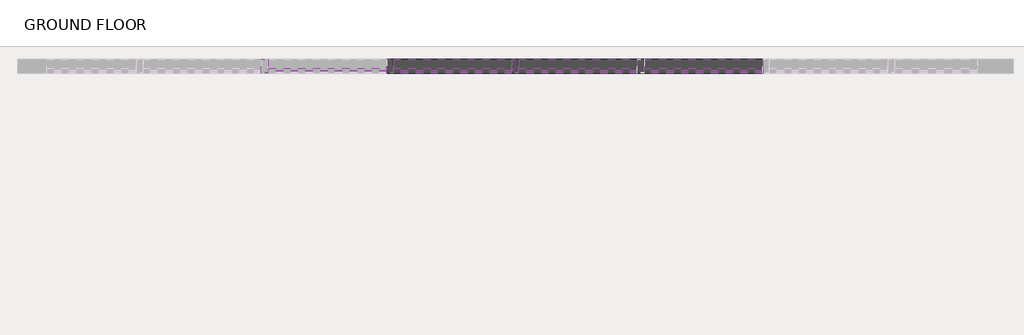
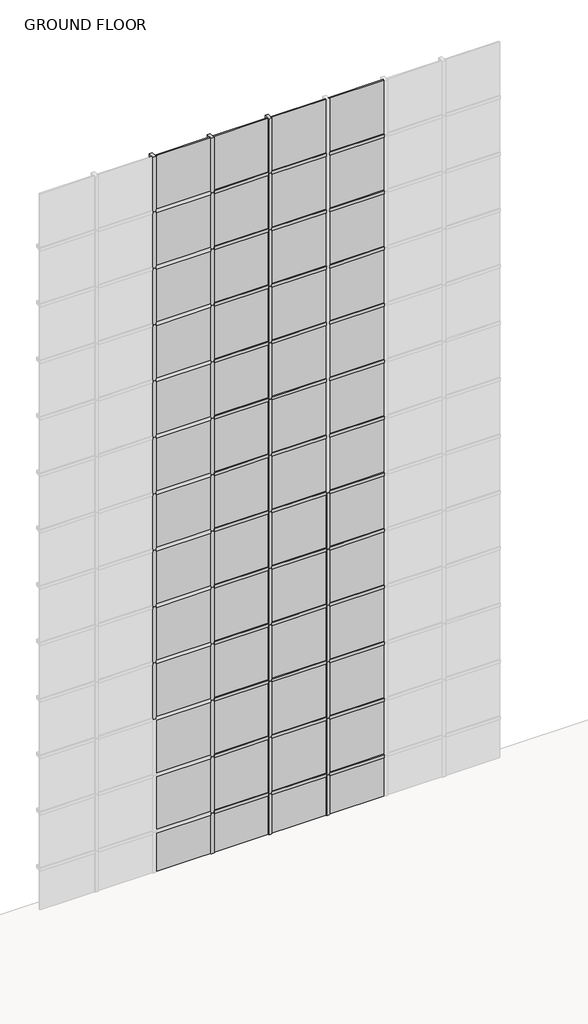
# One storey, part 10 of 16: 78 members, 52 plates.
"""IFC4 building model written with IfcOpenShell, lengths in millimetres."""

from ifc_helpers import new_model, si_unit, origin, place, context, project, spatial, transform, mapped, element, save
from components import member_d518c94e, member_b860638c, member_31fee25f, system_panel_glazed_5cba32e5

model = new_model("IFC4")

# Units and contexts
model_context = context("Model", 3, world=origin())
ifc_project = project(units=[si_unit("LENGTHUNIT", "METRE", prefix="MILLI")], contexts=[model_context])

# Site, building, storey
site = spatial("IfcSite", under=ifc_project)
building = spatial("IfcBuilding", under=site)
storey = spatial("IfcBuildingStorey", under=building, Name="GROUND FLOOR", Elevation=0.0)

# Members
placement = place(None, origin())
member_shape = member_d518c94e(model_context)
element("IfcMember", 1, ObjectType="Rectangular Mullion : 2.5\" x 5\" rectangular", at=placement, inside=storey, context=model_context, shape_type="MappedRepresentation", body=[
    mapped(member_shape, transform((-966.6171381, 6370.2261968, 1168.8884615), x_axis=(0.0, 0.0, 1.0), y_axis=(0.0, 1.0, 0.0), z_axis=(-1.0, 0.0, 0.0))),
])
element("IfcMember", 2, ObjectType="Rectangular Mullion : 2.5\" x 5\" rectangular", at=placement, inside=storey, context=model_context, shape_type="MappedRepresentation", body=[
    mapped(member_shape, transform((-2132.0863688, 6370.2261968, 1168.8884615), x_axis=(0.0, 0.0, 1.0), y_axis=(0.0, 1.0, 0.0), z_axis=(-1.0, 0.0, 0.0))),
])
element("IfcMember", 3, ObjectType="Rectangular Mullion : 2.5\" x 5\" rectangular", at=placement, inside=storey, context=model_context, shape_type="MappedRepresentation", body=[
    mapped(member_shape, transform((-3297.5555995, 6370.2261968, 1168.8884615), x_axis=(0.0, 0.0, 1.0), y_axis=(0.0, 1.0, 0.0), z_axis=(-1.0, 0.0, 0.0))),
])
element("IfcMember", 4, ObjectType="Rectangular Mullion : 2.5\" x 5\" rectangular", at=placement, inside=storey, context=model_context, shape_type="MappedRepresentation", body=[
    mapped(member_shape, transform((-966.6171381, 6370.2261968, 2369.5269231), x_axis=(0.0, 0.0, 1.0), y_axis=(0.0, 1.0, 0.0), z_axis=(-1.0, 0.0, 0.0))),
])
element("IfcMember", 5, ObjectType="Rectangular Mullion : 2.5\" x 5\" rectangular", at=placement, inside=storey, context=model_context, shape_type="MappedRepresentation", body=[
    mapped(member_shape, transform((-2132.0863688, 6370.2261968, 2369.5269231), x_axis=(0.0, 0.0, 1.0), y_axis=(0.0, 1.0, 0.0), z_axis=(-1.0, 0.0, 0.0))),
])
element("IfcMember", 6, ObjectType="Rectangular Mullion : 2.5\" x 5\" rectangular", at=placement, inside=storey, context=model_context, shape_type="MappedRepresentation", body=[
    mapped(member_shape, transform((-3297.5555995, 6370.2261968, 2369.5269231), x_axis=(0.0, 0.0, 1.0), y_axis=(0.0, 1.0, 0.0), z_axis=(-1.0, 0.0, 0.0))),
])
element("IfcMember", 7, ObjectType="Rectangular Mullion : 2.5\" x 5\" rectangular", at=placement, inside=storey, context=model_context, shape_type="MappedRepresentation", body=[
    mapped(member_shape, transform((-966.6171381, 6370.2261968, 3570.1653846), x_axis=(0.0, 0.0, 1.0), y_axis=(0.0, 1.0, 0.0), z_axis=(-1.0, 0.0, 0.0))),
])
element("IfcMember", 8, ObjectType="Rectangular Mullion : 2.5\" x 5\" rectangular", at=placement, inside=storey, context=model_context, shape_type="MappedRepresentation", body=[
    mapped(member_shape, transform((-2132.0863688, 6370.2261968, 3570.1653846), x_axis=(0.0, 0.0, 1.0), y_axis=(0.0, 1.0, 0.0), z_axis=(-1.0, 0.0, 0.0))),
])
element("IfcMember", 9, ObjectType="Rectangular Mullion : 2.5\" x 5\" rectangular", at=placement, inside=storey, context=model_context, shape_type="MappedRepresentation", body=[
    mapped(member_shape, transform((-3297.5555995, 6370.2261968, 3570.1653846), x_axis=(0.0, 0.0, 1.0), y_axis=(0.0, 1.0, 0.0), z_axis=(-1.0, 0.0, 0.0))),
])
element("IfcMember", 10, ObjectType="Rectangular Mullion : 2.5\" x 5\" rectangular", at=placement, inside=storey, context=model_context, shape_type="MappedRepresentation", body=[
    mapped(member_shape, transform((-966.6171381, 6370.2261968, 4770.8038462), x_axis=(0.0, 0.0, 1.0), y_axis=(0.0, 1.0, 0.0), z_axis=(-1.0, 0.0, 0.0))),
])
element("IfcMember", 11, ObjectType="Rectangular Mullion : 2.5\" x 5\" rectangular", at=placement, inside=storey, context=model_context, shape_type="MappedRepresentation", body=[
    mapped(member_shape, transform((-2132.0863688, 6370.2261968, 4770.8038462), x_axis=(0.0, 0.0, 1.0), y_axis=(0.0, 1.0, 0.0), z_axis=(-1.0, 0.0, 0.0))),
])
element("IfcMember", 12, ObjectType="Rectangular Mullion : 2.5\" x 5\" rectangular", at=placement, inside=storey, context=model_context, shape_type="MappedRepresentation", body=[
    mapped(member_shape, transform((-3297.5555995, 6370.2261968, 4770.8038462), x_axis=(0.0, 0.0, 1.0), y_axis=(0.0, 1.0, 0.0), z_axis=(-1.0, 0.0, 0.0))),
])
element("IfcMember", 13, ObjectType="Rectangular Mullion : 2.5\" x 5\" rectangular", at=placement, inside=storey, context=model_context, shape_type="MappedRepresentation", body=[
    mapped(member_shape, transform((-966.6171381, 6370.2261968, 5971.4423077), x_axis=(0.0, 0.0, 1.0), y_axis=(0.0, 1.0, 0.0), z_axis=(-1.0, 0.0, 0.0))),
])
element("IfcMember", 14, ObjectType="Rectangular Mullion : 2.5\" x 5\" rectangular", at=placement, inside=storey, context=model_context, shape_type="MappedRepresentation", body=[
    mapped(member_shape, transform((-2132.0863688, 6370.2261968, 5971.4423077), x_axis=(0.0, 0.0, 1.0), y_axis=(0.0, 1.0, 0.0), z_axis=(-1.0, 0.0, 0.0))),
])
element("IfcMember", 15, ObjectType="Rectangular Mullion : 2.5\" x 5\" rectangular", at=placement, inside=storey, context=model_context, shape_type="MappedRepresentation", body=[
    mapped(member_shape, transform((-3297.5555995, 6370.2261968, 5971.4423077), x_axis=(0.0, 0.0, 1.0), y_axis=(0.0, 1.0, 0.0), z_axis=(-1.0, 0.0, 0.0))),
])
element("IfcMember", 16, ObjectType="Rectangular Mullion : 2.5\" x 5\" rectangular", at=placement, inside=storey, context=model_context, shape_type="MappedRepresentation", body=[
    mapped(member_shape, transform((-966.6171381, 6370.2261968, 7172.0807692), x_axis=(0.0, 0.0, 1.0), y_axis=(0.0, 1.0, 0.0), z_axis=(-1.0, 0.0, 0.0))),
])
element("IfcMember", 17, ObjectType="Rectangular Mullion : 2.5\" x 5\" rectangular", at=placement, inside=storey, context=model_context, shape_type="MappedRepresentation", body=[
    mapped(member_shape, transform((-2132.0863688, 6370.2261968, 7172.0807692), x_axis=(0.0, 0.0, 1.0), y_axis=(0.0, 1.0, 0.0), z_axis=(-1.0, 0.0, 0.0))),
])
element("IfcMember", 18, ObjectType="Rectangular Mullion : 2.5\" x 5\" rectangular", at=placement, inside=storey, context=model_context, shape_type="MappedRepresentation", body=[
    mapped(member_shape, transform((-3297.5555995, 6370.2261968, 7172.0807692), x_axis=(0.0, 0.0, 1.0), y_axis=(0.0, 1.0, 0.0), z_axis=(-1.0, 0.0, 0.0))),
])
element("IfcMember", 19, ObjectType="Rectangular Mullion : 2.5\" x 5\" rectangular", at=placement, inside=storey, context=model_context, shape_type="MappedRepresentation", body=[
    mapped(member_shape, transform((-966.6171381, 6370.2261968, 8372.7192308), x_axis=(0.0, 0.0, 1.0), y_axis=(0.0, 1.0, 0.0), z_axis=(-1.0, 0.0, 0.0))),
])
element("IfcMember", 20, ObjectType="Rectangular Mullion : 2.5\" x 5\" rectangular", at=placement, inside=storey, context=model_context, shape_type="MappedRepresentation", body=[
    mapped(member_shape, transform((-2132.0863688, 6370.2261968, 8372.7192308), x_axis=(0.0, 0.0, 1.0), y_axis=(0.0, 1.0, 0.0), z_axis=(-1.0, 0.0, 0.0))),
])
element("IfcMember", 21, ObjectType="Rectangular Mullion : 2.5\" x 5\" rectangular", at=placement, inside=storey, context=model_context, shape_type="MappedRepresentation", body=[
    mapped(member_shape, transform((-3297.5555995, 6370.2261968, 8372.7192308), x_axis=(0.0, 0.0, 1.0), y_axis=(0.0, 1.0, 0.0), z_axis=(-1.0, 0.0, 0.0))),
])
element("IfcMember", 22, ObjectType="Rectangular Mullion : 2.5\" x 5\" rectangular", at=placement, inside=storey, context=model_context, shape_type="MappedRepresentation", body=[
    mapped(member_shape, transform((-966.6171381, 6370.2261968, 9573.3576923), x_axis=(0.0, 0.0, 1.0), y_axis=(0.0, 1.0, 0.0), z_axis=(-1.0, 0.0, 0.0))),
])
element("IfcMember", 23, ObjectType="Rectangular Mullion : 2.5\" x 5\" rectangular", at=placement, inside=storey, context=model_context, shape_type="MappedRepresentation", body=[
    mapped(member_shape, transform((-2132.0863688, 6370.2261968, 9573.3576923), x_axis=(0.0, 0.0, 1.0), y_axis=(0.0, 1.0, 0.0), z_axis=(-1.0, 0.0, 0.0))),
])
element("IfcMember", 24, ObjectType="Rectangular Mullion : 2.5\" x 5\" rectangular", at=placement, inside=storey, context=model_context, shape_type="MappedRepresentation", body=[
    mapped(member_shape, transform((-3297.5555995, 6370.2261968, 9573.3576923), x_axis=(0.0, 0.0, 1.0), y_axis=(0.0, 1.0, 0.0), z_axis=(-1.0, 0.0, 0.0))),
])
element("IfcMember", 25, ObjectType="Rectangular Mullion : 2.5\" x 5\" rectangular", at=placement, inside=storey, context=model_context, shape_type="MappedRepresentation", body=[
    mapped(member_shape, transform((-966.6171381, 6370.2261968, 10773.9961538), x_axis=(0.0, 0.0, 1.0), y_axis=(0.0, 1.0, 0.0), z_axis=(-1.0, 0.0, 0.0))),
])
element("IfcMember", 26, ObjectType="Rectangular Mullion : 2.5\" x 5\" rectangular", at=placement, inside=storey, context=model_context, shape_type="MappedRepresentation", body=[
    mapped(member_shape, transform((-2132.0863688, 6370.2261968, 10773.9961538), x_axis=(0.0, 0.0, 1.0), y_axis=(0.0, 1.0, 0.0), z_axis=(-1.0, 0.0, 0.0))),
])
element("IfcMember", 27, ObjectType="Rectangular Mullion : 2.5\" x 5\" rectangular", at=placement, inside=storey, context=model_context, shape_type="MappedRepresentation", body=[
    mapped(member_shape, transform((-3297.5555995, 6370.2261968, 10773.9961538), x_axis=(0.0, 0.0, 1.0), y_axis=(0.0, 1.0, 0.0), z_axis=(-1.0, 0.0, 0.0))),
])
element("IfcMember", 28, ObjectType="Rectangular Mullion : 2.5\" x 5\" rectangular", at=placement, inside=storey, context=model_context, shape_type="MappedRepresentation", body=[
    mapped(member_shape, transform((-966.6171381, 6370.2261968, 11974.6346154), x_axis=(0.0, 0.0, 1.0), y_axis=(0.0, 1.0, 0.0), z_axis=(-1.0, 0.0, 0.0))),
])
element("IfcMember", 29, ObjectType="Rectangular Mullion : 2.5\" x 5\" rectangular", at=placement, inside=storey, context=model_context, shape_type="MappedRepresentation", body=[
    mapped(member_shape, transform((-2132.0863688, 6370.2261968, 11974.6346154), x_axis=(0.0, 0.0, 1.0), y_axis=(0.0, 1.0, 0.0), z_axis=(-1.0, 0.0, 0.0))),
])
element("IfcMember", 30, ObjectType="Rectangular Mullion : 2.5\" x 5\" rectangular", at=placement, inside=storey, context=model_context, shape_type="MappedRepresentation", body=[
    mapped(member_shape, transform((-3297.5555995, 6370.2261968, 11974.6346154), x_axis=(0.0, 0.0, 1.0), y_axis=(0.0, 1.0, 0.0), z_axis=(-1.0, 0.0, 0.0))),
])
element("IfcMember", 31, ObjectType="Rectangular Mullion : 2.5\" x 5\" rectangular", at=placement, inside=storey, context=model_context, shape_type="MappedRepresentation", body=[
    mapped(member_shape, transform((-966.6171381, 6370.2261968, 13175.2730769), x_axis=(0.0, 0.0, 1.0), y_axis=(0.0, 1.0, 0.0), z_axis=(-1.0, 0.0, 0.0))),
])
element("IfcMember", 32, ObjectType="Rectangular Mullion : 2.5\" x 5\" rectangular", at=placement, inside=storey, context=model_context, shape_type="MappedRepresentation", body=[
    mapped(member_shape, transform((-2132.0863688, 6370.2261968, 13175.2730769), x_axis=(0.0, 0.0, 1.0), y_axis=(0.0, 1.0, 0.0), z_axis=(-1.0, 0.0, 0.0))),
])
element("IfcMember", 33, ObjectType="Rectangular Mullion : 2.5\" x 5\" rectangular", at=placement, inside=storey, context=model_context, shape_type="MappedRepresentation", body=[
    mapped(member_shape, transform((-3297.5555995, 6370.2261968, 13175.2730769), x_axis=(0.0, 0.0, 1.0), y_axis=(0.0, 1.0, 0.0), z_axis=(-1.0, 0.0, 0.0))),
])
element("IfcMember", 34, ObjectType="Rectangular Mullion : 2.5\" x 5\" rectangular", at=placement, inside=storey, context=model_context, shape_type="MappedRepresentation", body=[
    mapped(member_shape, transform((-966.6171381, 6370.2261968, 14375.9115385), x_axis=(0.0, 0.0, 1.0), y_axis=(0.0, 1.0, 0.0), z_axis=(-1.0, 0.0, 0.0))),
])
element("IfcMember", 35, ObjectType="Rectangular Mullion : 2.5\" x 5\" rectangular", at=placement, inside=storey, context=model_context, shape_type="MappedRepresentation", body=[
    mapped(member_shape, transform((-2132.0863688, 6370.2261968, 14375.9115385), x_axis=(0.0, 0.0, 1.0), y_axis=(0.0, 1.0, 0.0), z_axis=(-1.0, 0.0, 0.0))),
])
element("IfcMember", 36, ObjectType="Rectangular Mullion : 2.5\" x 5\" rectangular", at=placement, inside=storey, context=model_context, shape_type="MappedRepresentation", body=[
    mapped(member_shape, transform((-3297.5555995, 6370.2261968, 14375.9115385), x_axis=(0.0, 0.0, 1.0), y_axis=(0.0, 1.0, 0.0), z_axis=(-1.0, 0.0, 0.0))),
])
member_2_shape = member_b860638c(model_context)
element("IfcMember", 37, ObjectType="Rectangular Mullion : 2.5\" x 5\" rectangular", at=placement, inside=storey, context=model_context, shape_type="MappedRepresentation", body=[
    mapped(member_2_shape, transform((-998.3671381, 6370.2261968, 0.0), x_axis=(-1.0, 0.0, 0.0), y_axis=(0.0, 1.0, 0.0), z_axis=(0.0, 0.0, -1.0))),
])
element("IfcMember", 38, ObjectType="Rectangular Mullion : 2.5\" x 5\" rectangular", at=placement, inside=storey, context=model_context, shape_type="MappedRepresentation", body=[
    mapped(member_2_shape, transform((-2163.8363688, 6370.2261968, 0.0), x_axis=(-1.0, 0.0, 0.0), y_axis=(0.0, 1.0, 0.0), z_axis=(0.0, 0.0, -1.0))),
])
element("IfcMember", 39, ObjectType="Rectangular Mullion : 2.5\" x 5\" rectangular", at=placement, inside=storey, context=model_context, shape_type="MappedRepresentation", body=[
    mapped(member_2_shape, transform((-3329.3055995, 6370.2261968, 0.0), x_axis=(-1.0, 0.0, 0.0), y_axis=(0.0, 1.0, 0.0), z_axis=(0.0, 0.0, -1.0))),
])
member_3_shape = member_31fee25f(model_context)
element("IfcMember", 40, ObjectType="Rectangular Mullion : 2.5\" x 5\" rectangular", at=placement, inside=storey, context=model_context, shape_type="MappedRepresentation", body=[
    mapped(member_3_shape, transform((-998.3671381, 6370.2261968, 1168.8884615), x_axis=(-1.0, 0.0, 0.0), y_axis=(0.0, 1.0, 0.0), z_axis=(0.0, 0.0, -1.0))),
])
element("IfcMember", 41, ObjectType="Rectangular Mullion : 2.5\" x 5\" rectangular", at=placement, inside=storey, context=model_context, shape_type="MappedRepresentation", body=[
    mapped(member_3_shape, transform((-2163.8363688, 6370.2261968, 1168.8884615), x_axis=(-1.0, 0.0, 0.0), y_axis=(0.0, 1.0, 0.0), z_axis=(0.0, 0.0, -1.0))),
])
element("IfcMember", 42, ObjectType="Rectangular Mullion : 2.5\" x 5\" rectangular", at=placement, inside=storey, context=model_context, shape_type="MappedRepresentation", body=[
    mapped(member_3_shape, transform((-3329.3055995, 6370.2261968, 1168.8884615), x_axis=(-1.0, 0.0, 0.0), y_axis=(0.0, 1.0, 0.0), z_axis=(0.0, 0.0, -1.0))),
])
element("IfcMember", 43, ObjectType="Rectangular Mullion : 2.5\" x 5\" rectangular", at=placement, inside=storey, context=model_context, shape_type="MappedRepresentation", body=[
    mapped(member_3_shape, transform((-998.3671381, 6370.2261968, 2369.5269231), x_axis=(-1.0, 0.0, 0.0), y_axis=(0.0, 1.0, 0.0), z_axis=(0.0, 0.0, -1.0))),
])
element("IfcMember", 44, ObjectType="Rectangular Mullion : 2.5\" x 5\" rectangular", at=placement, inside=storey, context=model_context, shape_type="MappedRepresentation", body=[
    mapped(member_3_shape, transform((-2163.8363688, 6370.2261968, 2369.5269231), x_axis=(-1.0, 0.0, 0.0), y_axis=(0.0, 1.0, 0.0), z_axis=(0.0, 0.0, -1.0))),
])
element("IfcMember", 45, ObjectType="Rectangular Mullion : 2.5\" x 5\" rectangular", at=placement, inside=storey, context=model_context, shape_type="MappedRepresentation", body=[
    mapped(member_3_shape, transform((-3329.3055995, 6370.2261968, 2369.5269231), x_axis=(-1.0, 0.0, 0.0), y_axis=(0.0, 1.0, 0.0), z_axis=(0.0, 0.0, -1.0))),
])
element("IfcMember", 46, ObjectType="Rectangular Mullion : 2.5\" x 5\" rectangular", at=placement, inside=storey, context=model_context, shape_type="MappedRepresentation", body=[
    mapped(member_3_shape, transform((-998.3671381, 6370.2261968, 3570.1653846), x_axis=(-1.0, 0.0, 0.0), y_axis=(0.0, 1.0, 0.0), z_axis=(0.0, 0.0, -1.0))),
])
element("IfcMember", 47, ObjectType="Rectangular Mullion : 2.5\" x 5\" rectangular", at=placement, inside=storey, context=model_context, shape_type="MappedRepresentation", body=[
    mapped(member_3_shape, transform((-2163.8363688, 6370.2261968, 3570.1653846), x_axis=(-1.0, 0.0, 0.0), y_axis=(0.0, 1.0, 0.0), z_axis=(0.0, 0.0, -1.0))),
])
element("IfcMember", 48, ObjectType="Rectangular Mullion : 2.5\" x 5\" rectangular", at=placement, inside=storey, context=model_context, shape_type="MappedRepresentation", body=[
    mapped(member_3_shape, transform((-3329.3055995, 6370.2261968, 3570.1653846), x_axis=(-1.0, 0.0, 0.0), y_axis=(0.0, 1.0, 0.0), z_axis=(0.0, 0.0, -1.0))),
])
element("IfcMember", 49, ObjectType="Rectangular Mullion : 2.5\" x 5\" rectangular", at=placement, inside=storey, context=model_context, shape_type="MappedRepresentation", body=[
    mapped(member_3_shape, transform((-4494.7748302, 6370.2261968, 3570.1653846), x_axis=(-1.0, 0.0, 0.0), y_axis=(0.0, 1.0, 0.0), z_axis=(0.0, 0.0, -1.0))),
])
element("IfcMember", 50, ObjectType="Rectangular Mullion : 2.5\" x 5\" rectangular", at=placement, inside=storey, context=model_context, shape_type="MappedRepresentation", body=[
    mapped(member_3_shape, transform((-998.3671381, 6370.2261968, 4770.8038462), x_axis=(-1.0, 0.0, 0.0), y_axis=(0.0, 1.0, 0.0), z_axis=(0.0, 0.0, -1.0))),
])
element("IfcMember", 51, ObjectType="Rectangular Mullion : 2.5\" x 5\" rectangular", at=placement, inside=storey, context=model_context, shape_type="MappedRepresentation", body=[
    mapped(member_3_shape, transform((-2163.8363688, 6370.2261968, 4770.8038462), x_axis=(-1.0, 0.0, 0.0), y_axis=(0.0, 1.0, 0.0), z_axis=(0.0, 0.0, -1.0))),
])
element("IfcMember", 52, ObjectType="Rectangular Mullion : 2.5\" x 5\" rectangular", at=placement, inside=storey, context=model_context, shape_type="MappedRepresentation", body=[
    mapped(member_3_shape, transform((-3329.3055995, 6370.2261968, 4770.8038462), x_axis=(-1.0, 0.0, 0.0), y_axis=(0.0, 1.0, 0.0), z_axis=(0.0, 0.0, -1.0))),
])
element("IfcMember", 53, ObjectType="Rectangular Mullion : 2.5\" x 5\" rectangular", at=placement, inside=storey, context=model_context, shape_type="MappedRepresentation", body=[
    mapped(member_3_shape, transform((-4494.7748302, 6370.2261968, 4770.8038462), x_axis=(-1.0, 0.0, 0.0), y_axis=(0.0, 1.0, 0.0), z_axis=(0.0, 0.0, -1.0))),
])
element("IfcMember", 54, ObjectType="Rectangular Mullion : 2.5\" x 5\" rectangular", at=placement, inside=storey, context=model_context, shape_type="MappedRepresentation", body=[
    mapped(member_3_shape, transform((-998.3671381, 6370.2261968, 5971.4423077), x_axis=(-1.0, 0.0, 0.0), y_axis=(0.0, 1.0, 0.0), z_axis=(0.0, 0.0, -1.0))),
])
element("IfcMember", 55, ObjectType="Rectangular Mullion : 2.5\" x 5\" rectangular", at=placement, inside=storey, context=model_context, shape_type="MappedRepresentation", body=[
    mapped(member_3_shape, transform((-2163.8363688, 6370.2261968, 5971.4423077), x_axis=(-1.0, 0.0, 0.0), y_axis=(0.0, 1.0, 0.0), z_axis=(0.0, 0.0, -1.0))),
])
element("IfcMember", 56, ObjectType="Rectangular Mullion : 2.5\" x 5\" rectangular", at=placement, inside=storey, context=model_context, shape_type="MappedRepresentation", body=[
    mapped(member_3_shape, transform((-3329.3055995, 6370.2261968, 5971.4423077), x_axis=(-1.0, 0.0, 0.0), y_axis=(0.0, 1.0, 0.0), z_axis=(0.0, 0.0, -1.0))),
])
element("IfcMember", 57, ObjectType="Rectangular Mullion : 2.5\" x 5\" rectangular", at=placement, inside=storey, context=model_context, shape_type="MappedRepresentation", body=[
    mapped(member_3_shape, transform((-4494.7748302, 6370.2261968, 5971.4423077), x_axis=(-1.0, 0.0, 0.0), y_axis=(0.0, 1.0, 0.0), z_axis=(0.0, 0.0, -1.0))),
])
element("IfcMember", 58, ObjectType="Rectangular Mullion : 2.5\" x 5\" rectangular", at=placement, inside=storey, context=model_context, shape_type="MappedRepresentation", body=[
    mapped(member_3_shape, transform((-2163.8363688, 6370.2261968, 7172.0807692), x_axis=(-1.0, 0.0, 0.0), y_axis=(0.0, 1.0, 0.0), z_axis=(0.0, 0.0, -1.0))),
])
element("IfcMember", 59, ObjectType="Rectangular Mullion : 2.5\" x 5\" rectangular", at=placement, inside=storey, context=model_context, shape_type="MappedRepresentation", body=[
    mapped(member_3_shape, transform((-3329.3055995, 6370.2261968, 7172.0807692), x_axis=(-1.0, 0.0, 0.0), y_axis=(0.0, 1.0, 0.0), z_axis=(0.0, 0.0, -1.0))),
])
element("IfcMember", 60, ObjectType="Rectangular Mullion : 2.5\" x 5\" rectangular", at=placement, inside=storey, context=model_context, shape_type="MappedRepresentation", body=[
    mapped(member_3_shape, transform((-4494.7748302, 6370.2261968, 7172.0807692), x_axis=(-1.0, 0.0, 0.0), y_axis=(0.0, 1.0, 0.0), z_axis=(0.0, 0.0, -1.0))),
])
element("IfcMember", 61, ObjectType="Rectangular Mullion : 2.5\" x 5\" rectangular", at=placement, inside=storey, context=model_context, shape_type="MappedRepresentation", body=[
    mapped(member_3_shape, transform((-2163.8363688, 6370.2261968, 8372.7192308), x_axis=(-1.0, 0.0, 0.0), y_axis=(0.0, 1.0, 0.0), z_axis=(0.0, 0.0, -1.0))),
])
element("IfcMember", 62, ObjectType="Rectangular Mullion : 2.5\" x 5\" rectangular", at=placement, inside=storey, context=model_context, shape_type="MappedRepresentation", body=[
    mapped(member_3_shape, transform((-3329.3055995, 6370.2261968, 8372.7192308), x_axis=(-1.0, 0.0, 0.0), y_axis=(0.0, 1.0, 0.0), z_axis=(0.0, 0.0, -1.0))),
])
element("IfcMember", 63, ObjectType="Rectangular Mullion : 2.5\" x 5\" rectangular", at=placement, inside=storey, context=model_context, shape_type="MappedRepresentation", body=[
    mapped(member_3_shape, transform((-4494.7748302, 6370.2261968, 8372.7192308), x_axis=(-1.0, 0.0, 0.0), y_axis=(0.0, 1.0, 0.0), z_axis=(0.0, 0.0, -1.0))),
])
element("IfcMember", 64, ObjectType="Rectangular Mullion : 2.5\" x 5\" rectangular", at=placement, inside=storey, context=model_context, shape_type="MappedRepresentation", body=[
    mapped(member_3_shape, transform((-2163.8363688, 6370.2261968, 9573.3576923), x_axis=(-1.0, 0.0, 0.0), y_axis=(0.0, 1.0, 0.0), z_axis=(0.0, 0.0, -1.0))),
])
element("IfcMember", 65, ObjectType="Rectangular Mullion : 2.5\" x 5\" rectangular", at=placement, inside=storey, context=model_context, shape_type="MappedRepresentation", body=[
    mapped(member_3_shape, transform((-3329.3055995, 6370.2261968, 9573.3576923), x_axis=(-1.0, 0.0, 0.0), y_axis=(0.0, 1.0, 0.0), z_axis=(0.0, 0.0, -1.0))),
])
element("IfcMember", 66, ObjectType="Rectangular Mullion : 2.5\" x 5\" rectangular", at=placement, inside=storey, context=model_context, shape_type="MappedRepresentation", body=[
    mapped(member_3_shape, transform((-4494.7748302, 6370.2261968, 9573.3576923), x_axis=(-1.0, 0.0, 0.0), y_axis=(0.0, 1.0, 0.0), z_axis=(0.0, 0.0, -1.0))),
])
element("IfcMember", 67, ObjectType="Rectangular Mullion : 2.5\" x 5\" rectangular", at=placement, inside=storey, context=model_context, shape_type="MappedRepresentation", body=[
    mapped(member_3_shape, transform((-2163.8363688, 6370.2261968, 10773.9961538), x_axis=(-1.0, 0.0, 0.0), y_axis=(0.0, 1.0, 0.0), z_axis=(0.0, 0.0, -1.0))),
])
element("IfcMember", 68, ObjectType="Rectangular Mullion : 2.5\" x 5\" rectangular", at=placement, inside=storey, context=model_context, shape_type="MappedRepresentation", body=[
    mapped(member_3_shape, transform((-3329.3055995, 6370.2261968, 10773.9961538), x_axis=(-1.0, 0.0, 0.0), y_axis=(0.0, 1.0, 0.0), z_axis=(0.0, 0.0, -1.0))),
])
element("IfcMember", 69, ObjectType="Rectangular Mullion : 2.5\" x 5\" rectangular", at=placement, inside=storey, context=model_context, shape_type="MappedRepresentation", body=[
    mapped(member_3_shape, transform((-4494.7748302, 6370.2261968, 10773.9961538), x_axis=(-1.0, 0.0, 0.0), y_axis=(0.0, 1.0, 0.0), z_axis=(0.0, 0.0, -1.0))),
])
element("IfcMember", 70, ObjectType="Rectangular Mullion : 2.5\" x 5\" rectangular", at=placement, inside=storey, context=model_context, shape_type="MappedRepresentation", body=[
    mapped(member_3_shape, transform((-2163.8363688, 6370.2261968, 11974.6346154), x_axis=(-1.0, 0.0, 0.0), y_axis=(0.0, 1.0, 0.0), z_axis=(0.0, 0.0, -1.0))),
])
element("IfcMember", 71, ObjectType="Rectangular Mullion : 2.5\" x 5\" rectangular", at=placement, inside=storey, context=model_context, shape_type="MappedRepresentation", body=[
    mapped(member_3_shape, transform((-3329.3055995, 6370.2261968, 11974.6346154), x_axis=(-1.0, 0.0, 0.0), y_axis=(0.0, 1.0, 0.0), z_axis=(0.0, 0.0, -1.0))),
])
element("IfcMember", 72, ObjectType="Rectangular Mullion : 2.5\" x 5\" rectangular", at=placement, inside=storey, context=model_context, shape_type="MappedRepresentation", body=[
    mapped(member_3_shape, transform((-4494.7748302, 6370.2261968, 11974.6346154), x_axis=(-1.0, 0.0, 0.0), y_axis=(0.0, 1.0, 0.0), z_axis=(0.0, 0.0, -1.0))),
])
element("IfcMember", 73, ObjectType="Rectangular Mullion : 2.5\" x 5\" rectangular", at=placement, inside=storey, context=model_context, shape_type="MappedRepresentation", body=[
    mapped(member_3_shape, transform((-2163.8363688, 6370.2261968, 13175.2730769), x_axis=(-1.0, 0.0, 0.0), y_axis=(0.0, 1.0, 0.0), z_axis=(0.0, 0.0, -1.0))),
])
element("IfcMember", 74, ObjectType="Rectangular Mullion : 2.5\" x 5\" rectangular", at=placement, inside=storey, context=model_context, shape_type="MappedRepresentation", body=[
    mapped(member_3_shape, transform((-3329.3055995, 6370.2261968, 13175.2730769), x_axis=(-1.0, 0.0, 0.0), y_axis=(0.0, 1.0, 0.0), z_axis=(0.0, 0.0, -1.0))),
])
element("IfcMember", 75, ObjectType="Rectangular Mullion : 2.5\" x 5\" rectangular", at=placement, inside=storey, context=model_context, shape_type="MappedRepresentation", body=[
    mapped(member_3_shape, transform((-4494.7748302, 6370.2261968, 13175.2730769), x_axis=(-1.0, 0.0, 0.0), y_axis=(0.0, 1.0, 0.0), z_axis=(0.0, 0.0, -1.0))),
])
element("IfcMember", 76, ObjectType="Rectangular Mullion : 2.5\" x 5\" rectangular", at=placement, inside=storey, context=model_context, shape_type="MappedRepresentation", body=[
    mapped(member_2_shape, transform((-2163.8363688, 6370.2261968, 14375.9115385), x_axis=(-1.0, 0.0, 0.0), y_axis=(0.0, 1.0, 0.0), z_axis=(0.0, 0.0, -1.0))),
])
element("IfcMember", 77, ObjectType="Rectangular Mullion : 2.5\" x 5\" rectangular", at=placement, inside=storey, context=model_context, shape_type="MappedRepresentation", body=[
    mapped(member_2_shape, transform((-3329.3055995, 6370.2261968, 14375.9115385), x_axis=(-1.0, 0.0, 0.0), y_axis=(0.0, 1.0, 0.0), z_axis=(0.0, 0.0, -1.0))),
])
element("IfcMember", 78, ObjectType="Rectangular Mullion : 2.5\" x 5\" rectangular", at=placement, inside=storey, context=model_context, shape_type="MappedRepresentation", body=[
    mapped(member_2_shape, transform((-4494.7748302, 6370.2261968, 14375.9115385), x_axis=(-1.0, 0.0, 0.0), y_axis=(0.0, 1.0, 0.0), z_axis=(0.0, 0.0, -1.0))),
])

# Plates
system_panel_glazed_shape = system_panel_glazed_5cba32e5(model_context)
element("IfcPlate", 79, ObjectType="System Panel : Glazed", at=placement, inside=storey, context=model_context, shape_type="MappedRepresentation", body=[
    mapped(system_panel_glazed_shape, transform((-415.6325227, 6370.2261968, 0.0), x_axis=(-1.0, 0.0, 0.0), y_axis=(0.0, -1.0, 0.0), z_axis=(0.0, 0.0, 1.0))),
])
element("IfcPlate", 80, ObjectType="System Panel : Glazed", at=placement, inside=storey, context=model_context, shape_type="MappedRepresentation", body=[
    mapped(system_panel_glazed_shape, transform((-1581.1017534, 6370.2261968, 0.0), x_axis=(-1.0, 0.0, 0.0), y_axis=(0.0, -1.0, 0.0), z_axis=(0.0, 0.0, 1.0))),
])
element("IfcPlate", 81, ObjectType="System Panel : Glazed", at=placement, inside=storey, context=model_context, shape_type="MappedRepresentation", body=[
    mapped(system_panel_glazed_shape, transform((-2746.5709841, 6370.2261968, 0.0), x_axis=(-1.0, 0.0, 0.0), y_axis=(0.0, -1.0, 0.0), z_axis=(0.0, 0.0, 1.0))),
])
element("IfcPlate", 82, ObjectType="System Panel : Glazed", at=placement, inside=storey, context=model_context, shape_type="MappedRepresentation", body=[
    mapped(system_panel_glazed_shape, transform((-3912.0402149, 6370.2261968, 0.0), x_axis=(-1.0, 0.0, 0.0), y_axis=(0.0, -1.0, 0.0), z_axis=(0.0, 0.0, 1.0))),
])
element("IfcPlate", 83, ObjectType="System Panel : Glazed", at=placement, inside=storey, context=model_context, shape_type="MappedRepresentation", body=[
    mapped(system_panel_glazed_shape, transform((-415.6325227, 6370.2261968, 1200.6384615), x_axis=(-1.0, 0.0, 0.0), y_axis=(0.0, -1.0, 0.0), z_axis=(0.0, 0.0, 1.0))),
])
element("IfcPlate", 84, ObjectType="System Panel : Glazed", at=placement, inside=storey, context=model_context, shape_type="MappedRepresentation", body=[
    mapped(system_panel_glazed_shape, transform((-1581.1017534, 6370.2261968, 1200.6384615), x_axis=(-1.0, 0.0, 0.0), y_axis=(0.0, -1.0, 0.0), z_axis=(0.0, 0.0, 1.0))),
])
element("IfcPlate", 85, ObjectType="System Panel : Glazed", at=placement, inside=storey, context=model_context, shape_type="MappedRepresentation", body=[
    mapped(system_panel_glazed_shape, transform((-2746.5709841, 6370.2261968, 1200.6384615), x_axis=(-1.0, 0.0, 0.0), y_axis=(0.0, -1.0, 0.0), z_axis=(0.0, 0.0, 1.0))),
])
element("IfcPlate", 86, ObjectType="System Panel : Glazed", at=placement, inside=storey, context=model_context, shape_type="MappedRepresentation", body=[
    mapped(system_panel_glazed_shape, transform((-3912.0402149, 6370.2261968, 1200.6384615), x_axis=(-1.0, 0.0, 0.0), y_axis=(0.0, -1.0, 0.0), z_axis=(0.0, 0.0, 1.0))),
])
element("IfcPlate", 87, ObjectType="System Panel : Glazed", at=placement, inside=storey, context=model_context, shape_type="MappedRepresentation", body=[
    mapped(system_panel_glazed_shape, transform((-415.6325227, 6370.2261968, 2401.2769231), x_axis=(-1.0, 0.0, 0.0), y_axis=(0.0, -1.0, 0.0), z_axis=(0.0, 0.0, 1.0))),
])
element("IfcPlate", 88, ObjectType="System Panel : Glazed", at=placement, inside=storey, context=model_context, shape_type="MappedRepresentation", body=[
    mapped(system_panel_glazed_shape, transform((-1581.1017534, 6370.2261968, 2401.2769231), x_axis=(-1.0, 0.0, 0.0), y_axis=(0.0, -1.0, 0.0), z_axis=(0.0, 0.0, 1.0))),
])
element("IfcPlate", 89, ObjectType="System Panel : Glazed", at=placement, inside=storey, context=model_context, shape_type="MappedRepresentation", body=[
    mapped(system_panel_glazed_shape, transform((-2746.5709841, 6370.2261968, 2401.2769231), x_axis=(-1.0, 0.0, 0.0), y_axis=(0.0, -1.0, 0.0), z_axis=(0.0, 0.0, 1.0))),
])
element("IfcPlate", 90, ObjectType="System Panel : Glazed", at=placement, inside=storey, context=model_context, shape_type="MappedRepresentation", body=[
    mapped(system_panel_glazed_shape, transform((-3912.0402149, 6370.2261968, 2401.2769231), x_axis=(-1.0, 0.0, 0.0), y_axis=(0.0, -1.0, 0.0), z_axis=(0.0, 0.0, 1.0))),
])
element("IfcPlate", 91, ObjectType="System Panel : Glazed", at=placement, inside=storey, context=model_context, shape_type="MappedRepresentation", body=[
    mapped(system_panel_glazed_shape, transform((-415.6325227, 6370.2261968, 3601.9153846), x_axis=(-1.0, 0.0, 0.0), y_axis=(0.0, -1.0, 0.0), z_axis=(0.0, 0.0, 1.0))),
])
element("IfcPlate", 92, ObjectType="System Panel : Glazed", at=placement, inside=storey, context=model_context, shape_type="MappedRepresentation", body=[
    mapped(system_panel_glazed_shape, transform((-1581.1017534, 6370.2261968, 3601.9153846), x_axis=(-1.0, 0.0, 0.0), y_axis=(0.0, -1.0, 0.0), z_axis=(0.0, 0.0, 1.0))),
])
element("IfcPlate", 93, ObjectType="System Panel : Glazed", at=placement, inside=storey, context=model_context, shape_type="MappedRepresentation", body=[
    mapped(system_panel_glazed_shape, transform((-2746.5709841, 6370.2261968, 3601.9153846), x_axis=(-1.0, 0.0, 0.0), y_axis=(0.0, -1.0, 0.0), z_axis=(0.0, 0.0, 1.0))),
])
element("IfcPlate", 94, ObjectType="System Panel : Glazed", at=placement, inside=storey, context=model_context, shape_type="MappedRepresentation", body=[
    mapped(system_panel_glazed_shape, transform((-3912.0402149, 6370.2261968, 3601.9153846), x_axis=(-1.0, 0.0, 0.0), y_axis=(0.0, -1.0, 0.0), z_axis=(0.0, 0.0, 1.0))),
])
element("IfcPlate", 95, ObjectType="System Panel : Glazed", at=placement, inside=storey, context=model_context, shape_type="MappedRepresentation", body=[
    mapped(system_panel_glazed_shape, transform((-415.6325227, 6370.2261968, 4802.5538462), x_axis=(-1.0, 0.0, 0.0), y_axis=(0.0, -1.0, 0.0), z_axis=(0.0, 0.0, 1.0))),
])
element("IfcPlate", 96, ObjectType="System Panel : Glazed", at=placement, inside=storey, context=model_context, shape_type="MappedRepresentation", body=[
    mapped(system_panel_glazed_shape, transform((-1581.1017534, 6370.2261968, 4802.5538462), x_axis=(-1.0, 0.0, 0.0), y_axis=(0.0, -1.0, 0.0), z_axis=(0.0, 0.0, 1.0))),
])
element("IfcPlate", 97, ObjectType="System Panel : Glazed", at=placement, inside=storey, context=model_context, shape_type="MappedRepresentation", body=[
    mapped(system_panel_glazed_shape, transform((-2746.5709841, 6370.2261968, 4802.5538462), x_axis=(-1.0, 0.0, 0.0), y_axis=(0.0, -1.0, 0.0), z_axis=(0.0, 0.0, 1.0))),
])
element("IfcPlate", 98, ObjectType="System Panel : Glazed", at=placement, inside=storey, context=model_context, shape_type="MappedRepresentation", body=[
    mapped(system_panel_glazed_shape, transform((-3912.0402149, 6370.2261968, 4802.5538462), x_axis=(-1.0, 0.0, 0.0), y_axis=(0.0, -1.0, 0.0), z_axis=(0.0, 0.0, 1.0))),
])
element("IfcPlate", 99, ObjectType="System Panel : Glazed", at=placement, inside=storey, context=model_context, shape_type="MappedRepresentation", body=[
    mapped(system_panel_glazed_shape, transform((-415.6325227, 6370.2261968, 6003.1923077), x_axis=(-1.0, 0.0, 0.0), y_axis=(0.0, -1.0, 0.0), z_axis=(0.0, 0.0, 1.0))),
])
element("IfcPlate", 100, ObjectType="System Panel : Glazed", at=placement, inside=storey, context=model_context, shape_type="MappedRepresentation", body=[
    mapped(system_panel_glazed_shape, transform((-1581.1017534, 6370.2261968, 6003.1923077), x_axis=(-1.0, 0.0, 0.0), y_axis=(0.0, -1.0, 0.0), z_axis=(0.0, 0.0, 1.0))),
])
element("IfcPlate", 101, ObjectType="System Panel : Glazed", at=placement, inside=storey, context=model_context, shape_type="MappedRepresentation", body=[
    mapped(system_panel_glazed_shape, transform((-2746.5709841, 6370.2261968, 6003.1923077), x_axis=(-1.0, 0.0, 0.0), y_axis=(0.0, -1.0, 0.0), z_axis=(0.0, 0.0, 1.0))),
])
element("IfcPlate", 102, ObjectType="System Panel : Glazed", at=placement, inside=storey, context=model_context, shape_type="MappedRepresentation", body=[
    mapped(system_panel_glazed_shape, transform((-3912.0402149, 6370.2261968, 6003.1923077), x_axis=(-1.0, 0.0, 0.0), y_axis=(0.0, -1.0, 0.0), z_axis=(0.0, 0.0, 1.0))),
])
element("IfcPlate", 103, ObjectType="System Panel : Glazed", at=placement, inside=storey, context=model_context, shape_type="MappedRepresentation", body=[
    mapped(system_panel_glazed_shape, transform((-415.6325227, 6370.2261968, 7203.8307692), x_axis=(-1.0, 0.0, 0.0), y_axis=(0.0, -1.0, 0.0), z_axis=(0.0, 0.0, 1.0))),
])
element("IfcPlate", 104, ObjectType="System Panel : Glazed", at=placement, inside=storey, context=model_context, shape_type="MappedRepresentation", body=[
    mapped(system_panel_glazed_shape, transform((-1581.1017534, 6370.2261968, 7203.8307692), x_axis=(-1.0, 0.0, 0.0), y_axis=(0.0, -1.0, 0.0), z_axis=(0.0, 0.0, 1.0))),
])
element("IfcPlate", 105, ObjectType="System Panel : Glazed", at=placement, inside=storey, context=model_context, shape_type="MappedRepresentation", body=[
    mapped(system_panel_glazed_shape, transform((-2746.5709841, 6370.2261968, 7203.8307692), x_axis=(-1.0, 0.0, 0.0), y_axis=(0.0, -1.0, 0.0), z_axis=(0.0, 0.0, 1.0))),
])
element("IfcPlate", 106, ObjectType="System Panel : Glazed", at=placement, inside=storey, context=model_context, shape_type="MappedRepresentation", body=[
    mapped(system_panel_glazed_shape, transform((-3912.0402149, 6370.2261968, 7203.8307692), x_axis=(-1.0, 0.0, 0.0), y_axis=(0.0, -1.0, 0.0), z_axis=(0.0, 0.0, 1.0))),
])
element("IfcPlate", 107, ObjectType="System Panel : Glazed", at=placement, inside=storey, context=model_context, shape_type="MappedRepresentation", body=[
    mapped(system_panel_glazed_shape, transform((-415.6325227, 6370.2261968, 8404.4692308), x_axis=(-1.0, 0.0, 0.0), y_axis=(0.0, -1.0, 0.0), z_axis=(0.0, 0.0, 1.0))),
])
element("IfcPlate", 108, ObjectType="System Panel : Glazed", at=placement, inside=storey, context=model_context, shape_type="MappedRepresentation", body=[
    mapped(system_panel_glazed_shape, transform((-1581.1017534, 6370.2261968, 8404.4692308), x_axis=(-1.0, 0.0, 0.0), y_axis=(0.0, -1.0, 0.0), z_axis=(0.0, 0.0, 1.0))),
])
element("IfcPlate", 109, ObjectType="System Panel : Glazed", at=placement, inside=storey, context=model_context, shape_type="MappedRepresentation", body=[
    mapped(system_panel_glazed_shape, transform((-2746.5709841, 6370.2261968, 8404.4692308), x_axis=(-1.0, 0.0, 0.0), y_axis=(0.0, -1.0, 0.0), z_axis=(0.0, 0.0, 1.0))),
])
element("IfcPlate", 110, ObjectType="System Panel : Glazed", at=placement, inside=storey, context=model_context, shape_type="MappedRepresentation", body=[
    mapped(system_panel_glazed_shape, transform((-3912.0402149, 6370.2261968, 8404.4692308), x_axis=(-1.0, 0.0, 0.0), y_axis=(0.0, -1.0, 0.0), z_axis=(0.0, 0.0, 1.0))),
])
element("IfcPlate", 111, ObjectType="System Panel : Glazed", at=placement, inside=storey, context=model_context, shape_type="MappedRepresentation", body=[
    mapped(system_panel_glazed_shape, transform((-415.6325227, 6370.2261968, 9605.1076923), x_axis=(-1.0, 0.0, 0.0), y_axis=(0.0, -1.0, 0.0), z_axis=(0.0, 0.0, 1.0))),
])
element("IfcPlate", 112, ObjectType="System Panel : Glazed", at=placement, inside=storey, context=model_context, shape_type="MappedRepresentation", body=[
    mapped(system_panel_glazed_shape, transform((-1581.1017534, 6370.2261968, 9605.1076923), x_axis=(-1.0, 0.0, 0.0), y_axis=(0.0, -1.0, 0.0), z_axis=(0.0, 0.0, 1.0))),
])
element("IfcPlate", 113, ObjectType="System Panel : Glazed", at=placement, inside=storey, context=model_context, shape_type="MappedRepresentation", body=[
    mapped(system_panel_glazed_shape, transform((-2746.5709841, 6370.2261968, 9605.1076923), x_axis=(-1.0, 0.0, 0.0), y_axis=(0.0, -1.0, 0.0), z_axis=(0.0, 0.0, 1.0))),
])
element("IfcPlate", 114, ObjectType="System Panel : Glazed", at=placement, inside=storey, context=model_context, shape_type="MappedRepresentation", body=[
    mapped(system_panel_glazed_shape, transform((-3912.0402149, 6370.2261968, 9605.1076923), x_axis=(-1.0, 0.0, 0.0), y_axis=(0.0, -1.0, 0.0), z_axis=(0.0, 0.0, 1.0))),
])
element("IfcPlate", 115, ObjectType="System Panel : Glazed", at=placement, inside=storey, context=model_context, shape_type="MappedRepresentation", body=[
    mapped(system_panel_glazed_shape, transform((-415.6325227, 6370.2261968, 10805.7461538), x_axis=(-1.0, 0.0, 0.0), y_axis=(0.0, -1.0, 0.0), z_axis=(0.0, 0.0, 1.0))),
])
element("IfcPlate", 116, ObjectType="System Panel : Glazed", at=placement, inside=storey, context=model_context, shape_type="MappedRepresentation", body=[
    mapped(system_panel_glazed_shape, transform((-1581.1017534, 6370.2261968, 10805.7461538), x_axis=(-1.0, 0.0, 0.0), y_axis=(0.0, -1.0, 0.0), z_axis=(0.0, 0.0, 1.0))),
])
element("IfcPlate", 117, ObjectType="System Panel : Glazed", at=placement, inside=storey, context=model_context, shape_type="MappedRepresentation", body=[
    mapped(system_panel_glazed_shape, transform((-2746.5709841, 6370.2261968, 10805.7461538), x_axis=(-1.0, 0.0, 0.0), y_axis=(0.0, -1.0, 0.0), z_axis=(0.0, 0.0, 1.0))),
])
element("IfcPlate", 118, ObjectType="System Panel : Glazed", at=placement, inside=storey, context=model_context, shape_type="MappedRepresentation", body=[
    mapped(system_panel_glazed_shape, transform((-3912.0402149, 6370.2261968, 10805.7461538), x_axis=(-1.0, 0.0, 0.0), y_axis=(0.0, -1.0, 0.0), z_axis=(0.0, 0.0, 1.0))),
])
element("IfcPlate", 119, ObjectType="System Panel : Glazed", at=placement, inside=storey, context=model_context, shape_type="MappedRepresentation", body=[
    mapped(system_panel_glazed_shape, transform((-415.6325227, 6370.2261968, 12006.3846154), x_axis=(-1.0, 0.0, 0.0), y_axis=(0.0, -1.0, 0.0), z_axis=(0.0, 0.0, 1.0))),
])
element("IfcPlate", 120, ObjectType="System Panel : Glazed", at=placement, inside=storey, context=model_context, shape_type="MappedRepresentation", body=[
    mapped(system_panel_glazed_shape, transform((-1581.1017534, 6370.2261968, 12006.3846154), x_axis=(-1.0, 0.0, 0.0), y_axis=(0.0, -1.0, 0.0), z_axis=(0.0, 0.0, 1.0))),
])
element("IfcPlate", 121, ObjectType="System Panel : Glazed", at=placement, inside=storey, context=model_context, shape_type="MappedRepresentation", body=[
    mapped(system_panel_glazed_shape, transform((-2746.5709841, 6370.2261968, 12006.3846154), x_axis=(-1.0, 0.0, 0.0), y_axis=(0.0, -1.0, 0.0), z_axis=(0.0, 0.0, 1.0))),
])
element("IfcPlate", 122, ObjectType="System Panel : Glazed", at=placement, inside=storey, context=model_context, shape_type="MappedRepresentation", body=[
    mapped(system_panel_glazed_shape, transform((-3912.0402149, 6370.2261968, 12006.3846154), x_axis=(-1.0, 0.0, 0.0), y_axis=(0.0, -1.0, 0.0), z_axis=(0.0, 0.0, 1.0))),
])
element("IfcPlate", 123, ObjectType="System Panel : Glazed", at=placement, inside=storey, context=model_context, shape_type="MappedRepresentation", body=[
    mapped(system_panel_glazed_shape, transform((-415.6325227, 6370.2261968, 13207.0230769), x_axis=(-1.0, 0.0, 0.0), y_axis=(0.0, -1.0, 0.0), z_axis=(0.0, 0.0, 1.0))),
])
element("IfcPlate", 124, ObjectType="System Panel : Glazed", at=placement, inside=storey, context=model_context, shape_type="MappedRepresentation", body=[
    mapped(system_panel_glazed_shape, transform((-1581.1017534, 6370.2261968, 13207.0230769), x_axis=(-1.0, 0.0, 0.0), y_axis=(0.0, -1.0, 0.0), z_axis=(0.0, 0.0, 1.0))),
])
element("IfcPlate", 125, ObjectType="System Panel : Glazed", at=placement, inside=storey, context=model_context, shape_type="MappedRepresentation", body=[
    mapped(system_panel_glazed_shape, transform((-2746.5709841, 6370.2261968, 13207.0230769), x_axis=(-1.0, 0.0, 0.0), y_axis=(0.0, -1.0, 0.0), z_axis=(0.0, 0.0, 1.0))),
])
element("IfcPlate", 126, ObjectType="System Panel : Glazed", at=placement, inside=storey, context=model_context, shape_type="MappedRepresentation", body=[
    mapped(system_panel_glazed_shape, transform((-3912.0402149, 6370.2261968, 13207.0230769), x_axis=(-1.0, 0.0, 0.0), y_axis=(0.0, -1.0, 0.0), z_axis=(0.0, 0.0, 1.0))),
])
element("IfcPlate", 127, ObjectType="System Panel : Glazed", at=placement, inside=storey, context=model_context, shape_type="MappedRepresentation", body=[
    mapped(system_panel_glazed_shape, transform((-415.6325227, 6370.2261968, 14407.6615385), x_axis=(-1.0, 0.0, 0.0), y_axis=(0.0, -1.0, 0.0), z_axis=(0.0, 0.0, 1.0))),
])
element("IfcPlate", 128, ObjectType="System Panel : Glazed", at=placement, inside=storey, context=model_context, shape_type="MappedRepresentation", body=[
    mapped(system_panel_glazed_shape, transform((-1581.1017534, 6370.2261968, 14407.6615385), x_axis=(-1.0, 0.0, 0.0), y_axis=(0.0, -1.0, 0.0), z_axis=(0.0, 0.0, 1.0))),
])
element("IfcPlate", 129, ObjectType="System Panel : Glazed", at=placement, inside=storey, context=model_context, shape_type="MappedRepresentation", body=[
    mapped(system_panel_glazed_shape, transform((-2746.5709841, 6370.2261968, 14407.6615385), x_axis=(-1.0, 0.0, 0.0), y_axis=(0.0, -1.0, 0.0), z_axis=(0.0, 0.0, 1.0))),
])
element("IfcPlate", 130, ObjectType="System Panel : Glazed", at=placement, inside=storey, context=model_context, shape_type="MappedRepresentation", body=[
    mapped(system_panel_glazed_shape, transform((-3912.0402149, 6370.2261968, 14407.6615385), x_axis=(-1.0, 0.0, 0.0), y_axis=(0.0, -1.0, 0.0), z_axis=(0.0, 0.0, 1.0))),
])

save(model, "model.ifc")

# Revit data of these elements
# Type "Rectangular Mullion : 2.5\" x 5\" rectangular"
#   built-in parameter 1007304 = 0.416667 (stored number, unit not read)
#   built-in parameter 1007301 = 0.104167 (stored number, unit not read)
#   built-in parameter 1007300 = 0.104167 (stored number, unit not read)
# Type "System Panel : Glazed"
#   Construction Type Id = "GSP4R"
#   Analytic Construction = "1/8 in Pilkington single glazing"
#   Visual Light Transmittance = 0.9
#   Solar Heat Gain Coefficient = 0.86
#   Heat Transfer Coefficient (U) = 1.18115 BTU/(h·ft²·°F)
#   Define Thermal Properties by = 1
# Elements 1, 2, 3, 4, 5, 6, 7, 8, 9, 10, 11, 12, 13, 14, 15, 16, 17, 18, 19, 20, 21, 22, 23, 24, 25, 26, 27, 28, 29, 30, 31, 32, 33, 34, 35, 36, 37, 38, 39, 40, 41, 42, 43, 44, 45, 46, 47, 48, 49, 50, 51, 52, 53, 54, 55, 56, 57, 58, 59, 60, 61, 62, 63, 64, 65, 66, 67, 68, 69, 70, 71, 72, 73, 74, 75, 76, 77, 78 (IfcMember, "Rectangular Mullion : 2.5\" x 5\" rectangular")
#   Phase Created = New Construction
#   Materials on its faces: "Aluminum"
# Elements 79, 80, 81, 82, 83, 84, 85, 86, 87, 88, 89, 90, 91, 92, 93, 94, 95, 96, 97, 98, 99, 100, 101, 102, 103, 104, 105, 106, 107, 108, 109, 110, 111, 112, 113, 114, 115, 116, 117, 118, 119, 120, 121, 122, 123, 124, 125, 126, 127, 128, 129, 130 (IfcPlate, "System Panel : Glazed")
#   Phase Created = New Construction
#   Materials on its faces: "Glass"
# Materials
#   "Aluminum": class "Metal", colour RGB 247 247 247, transparency 0, Description = "Aluminum 6061", Cost = 0
#   "Glass": class "Glass", colour RGB 0 128 192, transparency 0.75, Description = "Soda Lime Glass", Cost = 0
